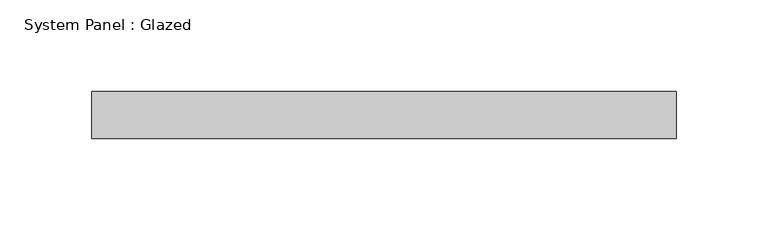
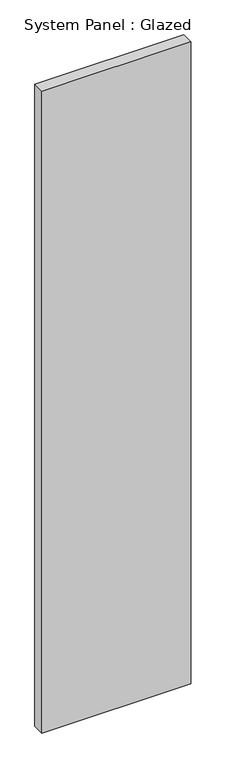
"""IFC4 building model written with IfcOpenShell, lengths in millimetres: plate geometry, System Panel : Glazed."""

from ifc_helpers import new_model, si_unit, origin, origin_with_axes, place, context, project, spatial, polyline, outline, extrude, source, transform, mapped, element, save


def system_panel_glazed_37470fb4(model_context):
    return source(origin(), model_context, "Body", "SweptSolid", [
        extrude(outline(polyline([(158.75, 19.05), (-158.75, 19.05), (-158.75, 44.45), (158.75, 44.45), (158.75, 19.05)])), origin_with_axes(), (0.0, 0.0, 1.0), 1447.2288132),
    ])


if __name__ == "__main__":
    model = new_model("IFC4")
    model_context = context("Model", 3, world=origin())
    ifc_project = project(units=[si_unit("LENGTHUNIT", "METRE", prefix="MILLI")], contexts=[model_context])
    site = spatial("IfcSite", under=ifc_project)
    building = spatial("IfcBuilding", under=site)
    placement = place(None, origin())
    system_panel_glazed_shape = system_panel_glazed_37470fb4(model_context)
    element("IfcPlate", 1, ObjectType="System Panel : Glazed", at=placement, inside=building, context=model_context, shape_type="MappedRepresentation", body=[
        mapped(system_panel_glazed_shape, transform((0.0, 0.0, 0.0), x_axis=(1.0, 0.0, 0.0), y_axis=(0.0, 1.0, 0.0), z_axis=(0.0, 0.0, 1.0))),
    ])
    save(model, "model.ifc")

# Revit data of these elements
# Type "System Panel : Glazed"
#   Construction Type Id = "GSP4R"
#   Analytic Construction = "1/8 in Pilkington single glazing"
#   Visual Light Transmittance = 0.9
#   Solar Heat Gain Coefficient = 0.86
#   Heat Transfer Coefficient (U) = 1.18115 BTU/(h·ft²·°F)
#   Define Thermal Properties by = 1
# Element 1 (IfcPlate, "System Panel : Glazed")
#   Materials on its faces: "Glass"
# Materials
#   "Glass": class "Glass", colour RGB 0 128 192, transparency 0.75, Description = "Soda Lime Glass", Cost = 0
